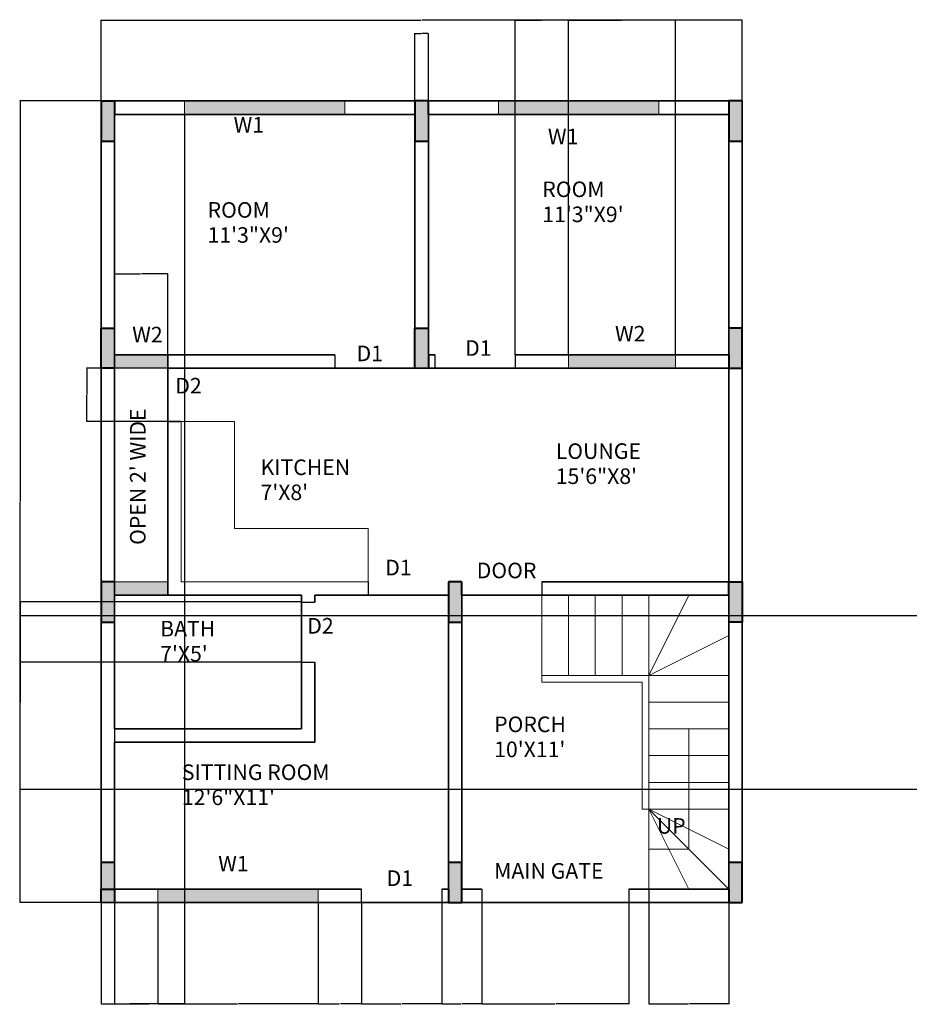
# Model space of a CAD drawing. Units: millimetres. Extents: x 1831 to 2754, y 1517 to 2450.
# Tile 1 of 4: x 1955 to 2355, y 1517 to 1959. Entities that reach past the tile are written whole.
import ezdxf

# ---------------------------------------------------------------- set-up
doc = ezdxf.new("R2010")
doc.units = ezdxf.units.MM
for name, color, linetype, lineweight in [('A-ANNO-DIMS', 2, 'Continuous', 18), ('A-ANNO-TEXT', 7, 'Continuous', 18), ('A-AREA-IDEN', 7, 'Continuous', 18), ('A-COLS', 7, 'Continuous', 40), ('A-DETL-REFP', 8, 'Continuous', 13), ('A-DOOR', 3, 'Continuous', 25), ('A-FLOR-CASE', 8, 'Continuous', 18), ('A-FLOR-STRS', 7, 'Continuous', 18), ('A-GLAZ', 4, 'Continuous', 18), ('A-WALL', 7, 'Continuous', 35)]:
    doc.layers.add(name, color=color, linetype=linetype, lineweight=lineweight)
doc.layers.add('A-COLS-PATT', color=18, linetype='Continuous', lineweight=13, true_color=0x000000)
doc.layers.add('A-GLAZ-PATT', color=252, linetype='Continuous', lineweight=13, true_color=0x939598)
doc.styles.get("Standard").update_dxf_attribs({"font": 'arial.ttf'})
doc.dimstyles.get("Standard").update_dxf_attribs({"dimtxt": 0.18, "dimasz": 0.18, "dimexe": 0.18, "dimexo": 0.0625, "dimgap": 0.09, "dimtad": 0, "dimtih": 1, "dimtoh": 1, "dimdec": 4, "dimzin": 0, "dimdsep": 46, "dimtxsty": 'Standard', "dimcen": 0.09, "dimadec": 0, "dimazin": 0, "dimtfac": 1, "dimtdec": 4, "dimtofl": 0, "dimtmove": 0, "dimatfit": 3, "dimfxl": 1, "dimtolj": 1, "dimtzin": 0, "dimarcsym": 0})

# ---------------------------------------------------------------- blocks, each defined once
blk = doc.blocks.new('*D22')
at = {"layer": 'A-ANNO-DIMS', "color": 0, "lineweight": -2, "transparency": 16777216}
for p, q in [((1991.57, 1922.44), (1991.57, 1958.89)), ((2279.57, 1922.44), (2279.57, 1958.89)), ((1991.75, 1958.71), (2135.28, 1958.71)), ((2279.39, 1958.71), (2135.86, 1958.71))]:
    blk.add_line(p, q, dxfattribs=at)
at = {"layer": 'A-ANNO-DIMS', "color": 0, "transparency": 16777216}
for points in [[(1991.75, 1958.74), (1991.75, 1958.68), (1991.57, 1958.71)], [(2279.39, 1958.74), (2279.39, 1958.68), (2279.57, 1958.71)]]:
    blk.add_solid(points, dxfattribs=at)
at = {"layer": 'Defpoints', "color": 0, "transparency": 16777216}
for p in [(2279.57, 1958.71), (1991.57, 1922.38), (2279.57, 1922.38)]:
    blk.add_point(p, dxfattribs=at)
at = {"layer": 'A-ANNO-DIMS', "color": 0, "transparency": 16777216, "insert": (2135.57, 1958.71), "char_height": 0.18, "attachment_point": 5}
blk.add_mtext('\\A1;288', dxfattribs=at)
blk = doc.blocks.new('*D23')
at = {"layer": 'A-ANNO-DIMS', "color": 0, "lineweight": -2, "transparency": 16777216}
for p, q in [((1991.51, 1922.38), (1955.06, 1922.38)), ((1955.24, 1922.2), (1955.24, 1742.56)), ((1955.24, 1562.56), (1955.24, 1742.2)), ((1991.51, 1562.38), (1955.06, 1562.38))]:
    blk.add_line(p, q, dxfattribs=at)
at = {"layer": 'A-ANNO-DIMS', "color": 0, "transparency": 16777216}
for points in [[(1955.21, 1922.2), (1955.27, 1922.2), (1955.24, 1922.38)], [(1955.21, 1562.56), (1955.27, 1562.56), (1955.24, 1562.38)]]:
    blk.add_solid(points, dxfattribs=at)
at = {"layer": 'Defpoints', "color": 0, "transparency": 16777216}
for p in [(1955.24, 1922.38), (1991.57, 1922.38), (1991.57, 1562.38)]:
    blk.add_point(p, dxfattribs=at)
at = {"layer": 'A-ANNO-DIMS', "color": 0, "transparency": 16777216, "insert": (1955.24, 1742.38), "char_height": 0.18, "attachment_point": 5}
blk.add_mtext('\\A1;360', dxfattribs=at)
blk = doc.blocks.new('*D24')
at = {"layer": 'A-ANNO-DIMS', "color": 0, "lineweight": -2, "transparency": 16777216}
for p, q in [((1991.57, 1562.32), (1991.57, 1516.71)), ((2017.07, 1562.32), (2017.07, 1516.71)), ((1991.75, 1516.89), (2003.99, 1516.89)), ((2016.89, 1516.89), (2004.64, 1516.89))]:
    blk.add_line(p, q, dxfattribs=at)
at = {"layer": 'A-ANNO-DIMS', "color": 0, "transparency": 16777216}
for points in [[(1991.75, 1516.92), (1991.75, 1516.86), (1991.57, 1516.89)], [(2016.89, 1516.92), (2016.89, 1516.86), (2017.07, 1516.89)]]:
    blk.add_solid(points, dxfattribs=at)
at = {"layer": 'Defpoints', "color": 0, "transparency": 16777216}
for p in [(1991.57, 1562.38), (2017.07, 1562.38), (2017.07, 1516.89)]:
    blk.add_point(p, dxfattribs=at)
at = {"layer": 'A-ANNO-DIMS', "color": 0, "transparency": 16777216, "insert": (2004.32, 1516.89), "char_height": 0.18, "attachment_point": 5}
blk.add_mtext('\\A1;25.5', dxfattribs=at)
blk = doc.blocks.new('*D25')
at = {"layer": 'A-ANNO-DIMS', "color": 0, "lineweight": -2, "transparency": 16777216}
for p, q in [((2017.07, 1562.32), (2017.07, 1516.71)), ((2089.07, 1562.32), (2089.07, 1516.71)), ((2017.25, 1516.89), (2052.85, 1516.89)), ((2088.89, 1516.89), (2053.29, 1516.89))]:
    blk.add_line(p, q, dxfattribs=at)
at = {"layer": 'A-ANNO-DIMS', "color": 0, "transparency": 16777216}
for points in [[(2017.25, 1516.92), (2017.25, 1516.86), (2017.07, 1516.89)], [(2088.89, 1516.92), (2088.89, 1516.86), (2089.07, 1516.89)]]:
    blk.add_solid(points, dxfattribs=at)
at = {"layer": 'Defpoints', "color": 0, "transparency": 16777216}
for p in [(2017.07, 1562.38), (2089.07, 1562.38), (2089.07, 1516.89)]:
    blk.add_point(p, dxfattribs=at)
at = {"layer": 'A-ANNO-DIMS', "color": 0, "transparency": 16777216, "insert": (2053.07, 1516.89), "char_height": 0.18, "attachment_point": 5}
blk.add_mtext('\\A1;72', dxfattribs=at)
blk = doc.blocks.new('*D26')
at = {"layer": 'A-ANNO-DIMS', "color": 0, "lineweight": -2, "transparency": 16777216}
for p, q in [((2089.07, 1562.32), (2089.07, 1516.71)), ((2108.57, 1562.32), (2108.57, 1516.71)), ((2089.25, 1516.89), (2098.5, 1516.89)), ((2108.39, 1516.89), (2099.13, 1516.89))]:
    blk.add_line(p, q, dxfattribs=at)
at = {"layer": 'A-ANNO-DIMS', "color": 0, "transparency": 16777216}
for points in [[(2089.25, 1516.92), (2089.25, 1516.86), (2089.07, 1516.89)], [(2108.39, 1516.92), (2108.39, 1516.86), (2108.57, 1516.89)]]:
    blk.add_solid(points, dxfattribs=at)
at = {"layer": 'Defpoints', "color": 0, "transparency": 16777216}
for p in [(2089.07, 1562.38), (2108.57, 1562.38), (2108.57, 1516.89)]:
    blk.add_point(p, dxfattribs=at)
at = {"layer": 'A-ANNO-DIMS', "color": 0, "transparency": 16777216, "insert": (2098.82, 1516.89), "char_height": 0.18, "attachment_point": 5}
blk.add_mtext('\\A1;19.5', dxfattribs=at)
blk = doc.blocks.new('*D27')
at = {"layer": 'A-ANNO-DIMS', "color": 0, "lineweight": -2, "transparency": 16777216}
for p, q in [((2108.57, 1562.32), (2108.57, 1516.71)), ((2144.57, 1562.32), (2144.57, 1516.71)), ((2108.75, 1516.89), (2126.35, 1516.89)), ((2144.39, 1516.89), (2126.79, 1516.89))]:
    blk.add_line(p, q, dxfattribs=at)
at = {"layer": 'A-ANNO-DIMS', "color": 0, "transparency": 16777216}
for points in [[(2108.75, 1516.92), (2108.75, 1516.86), (2108.57, 1516.89)], [(2144.39, 1516.92), (2144.39, 1516.86), (2144.57, 1516.89)]]:
    blk.add_solid(points, dxfattribs=at)
at = {"layer": 'Defpoints', "color": 0, "transparency": 16777216}
for p in [(2108.57, 1562.38), (2144.57, 1562.38), (2144.57, 1516.89)]:
    blk.add_point(p, dxfattribs=at)
at = {"layer": 'A-ANNO-DIMS', "color": 0, "transparency": 16777216, "insert": (2126.57, 1516.89), "char_height": 0.18, "attachment_point": 5}
blk.add_mtext('\\A1;36', dxfattribs=at)
blk = doc.blocks.new('*D28')
at = {"layer": 'A-ANNO-DIMS', "color": 0, "lineweight": -2, "transparency": 16777216}
for p, q in [((2144.57, 1562.32), (2144.57, 1516.71)), ((2162.57, 1562.32), (2162.57, 1516.71)), ((2144.75, 1516.89), (2153.36, 1516.89)), ((2162.39, 1516.89), (2153.78, 1516.89))]:
    blk.add_line(p, q, dxfattribs=at)
at = {"layer": 'A-ANNO-DIMS', "color": 0, "transparency": 16777216}
for points in [[(2144.75, 1516.92), (2144.75, 1516.86), (2144.57, 1516.89)], [(2162.39, 1516.92), (2162.39, 1516.86), (2162.57, 1516.89)]]:
    blk.add_solid(points, dxfattribs=at)
at = {"layer": 'Defpoints', "color": 0, "transparency": 16777216}
for p in [(2144.57, 1562.38), (2162.57, 1562.38), (2162.57, 1516.89)]:
    blk.add_point(p, dxfattribs=at)
at = {"layer": 'A-ANNO-DIMS', "color": 0, "transparency": 16777216, "insert": (2153.57, 1516.89), "char_height": 0.18, "attachment_point": 5}
blk.add_mtext('\\A1;18', dxfattribs=at)
blk = doc.blocks.new('*D29')
at = {"layer": 'A-ANNO-DIMS', "color": 0, "lineweight": -2, "transparency": 16777216}
for p, q in [((2162.57, 1562.32), (2162.57, 1516.71)), ((2228.57, 1562.32), (2228.57, 1516.71)), ((2162.75, 1516.89), (2195.35, 1516.89)), ((2228.39, 1516.89), (2195.79, 1516.89))]:
    blk.add_line(p, q, dxfattribs=at)
at = {"layer": 'A-ANNO-DIMS', "color": 0, "transparency": 16777216}
for points in [[(2162.75, 1516.92), (2162.75, 1516.86), (2162.57, 1516.89)], [(2228.39, 1516.92), (2228.39, 1516.86), (2228.57, 1516.89)]]:
    blk.add_solid(points, dxfattribs=at)
at = {"layer": 'Defpoints', "color": 0, "transparency": 16777216}
for p in [(2162.57, 1562.38), (2228.57, 1562.38), (2228.57, 1516.89)]:
    blk.add_point(p, dxfattribs=at)
at = {"layer": 'A-ANNO-DIMS', "color": 0, "transparency": 16777216, "insert": (2195.57, 1516.89), "char_height": 0.18, "attachment_point": 5}
blk.add_mtext('\\A1;66', dxfattribs=at)
blk = doc.blocks.new('*D30')
at = {"layer": 'A-ANNO-DIMS', "color": 0, "lineweight": -2, "transparency": 16777216}
for p, q in [((1997.57, 1916.32), (1997.57, 1516.71)), ((2029.07, 1916.32), (2029.07, 1516.71)), ((1997.75, 1516.89), (2012.99, 1516.89)), ((2028.89, 1516.89), (2013.64, 1516.89))]:
    blk.add_line(p, q, dxfattribs=at)
at = {"layer": 'A-ANNO-DIMS', "color": 0, "transparency": 16777216}
for points in [[(1997.75, 1516.92), (1997.75, 1516.86), (1997.57, 1516.89)], [(2028.89, 1516.92), (2028.89, 1516.86), (2029.07, 1516.89)]]:
    blk.add_solid(points, dxfattribs=at)
at = {"layer": 'Defpoints', "color": 0, "transparency": 16777216}
for p in [(1997.57, 1916.38), (2029.07, 1916.38), (2029.07, 1516.89)]:
    blk.add_point(p, dxfattribs=at)
at = {"layer": 'A-ANNO-DIMS', "color": 0, "transparency": 16777216, "insert": (2013.32, 1516.89), "char_height": 0.18, "attachment_point": 5}
blk.add_mtext('\\A1;31.5', dxfattribs=at)
blk = doc.blocks.new('*D31')
at = {"layer": 'A-ANNO-DIMS', "color": 0, "lineweight": -2, "transparency": 16777216}
for p, q in [((2177.57, 1808.44), (2177.57, 1958.89)), ((2201.57, 1808.44), (2201.57, 1958.89)), ((2177.75, 1958.71), (2189.35, 1958.71)), ((2201.39, 1958.71), (2189.79, 1958.71))]:
    blk.add_line(p, q, dxfattribs=at)
at = {"layer": 'A-ANNO-DIMS', "color": 0, "transparency": 16777216}
for points in [[(2177.75, 1958.74), (2177.75, 1958.68), (2177.57, 1958.71)], [(2201.39, 1958.74), (2201.39, 1958.68), (2201.57, 1958.71)]]:
    blk.add_solid(points, dxfattribs=at)
at = {"layer": 'Defpoints', "color": 0, "transparency": 16777216}
for p in [(2201.57, 1958.71), (2177.57, 1808.38), (2201.57, 1808.38)]:
    blk.add_point(p, dxfattribs=at)
at = {"layer": 'A-ANNO-DIMS', "color": 0, "transparency": 16777216, "insert": (2189.57, 1958.71), "char_height": 0.18, "attachment_point": 5}
blk.add_mtext('\\A1;24', dxfattribs=at)
blk = doc.blocks.new('*D32')
at = {"layer": 'A-ANNO-DIMS', "color": 0, "lineweight": -2, "transparency": 16777216}
for p, q in [((2201.57, 1808.44), (2201.57, 1958.89)), ((2249.57, 1808.44), (2249.57, 1958.89)), ((2201.75, 1958.71), (2225.35, 1958.71)), ((2249.39, 1958.71), (2225.79, 1958.71))]:
    blk.add_line(p, q, dxfattribs=at)
at = {"layer": 'A-ANNO-DIMS', "color": 0, "transparency": 16777216}
for points in [[(2201.75, 1958.74), (2201.75, 1958.68), (2201.57, 1958.71)], [(2249.39, 1958.74), (2249.39, 1958.68), (2249.57, 1958.71)]]:
    blk.add_solid(points, dxfattribs=at)
at = {"layer": 'Defpoints', "color": 0, "transparency": 16777216}
for p in [(2249.57, 1958.71), (2201.57, 1808.38), (2249.57, 1808.38)]:
    blk.add_point(p, dxfattribs=at)
at = {"layer": 'A-ANNO-DIMS', "color": 0, "transparency": 16777216, "insert": (2225.57, 1958.71), "char_height": 0.18, "attachment_point": 5}
blk.add_mtext('\\A1;48', dxfattribs=at)
blk = doc.blocks.new('*D33')
at = {"layer": 'A-ANNO-DIMS', "color": 0, "lineweight": -2, "transparency": 16777216}
for p, q in [((1997.57, 1808.44), (1997.57, 1844.89)), ((1997.75, 1844.71), (2009.35, 1844.71)), ((2021.39, 1844.71), (2009.79, 1844.71)), ((2021.57, 1808.44), (2021.57, 1844.89))]:
    blk.add_line(p, q, dxfattribs=at)
at = {"layer": 'A-ANNO-DIMS', "color": 0, "transparency": 16777216}
for points in [[(1997.75, 1844.74), (1997.75, 1844.68), (1997.57, 1844.71)], [(2021.39, 1844.74), (2021.39, 1844.68), (2021.57, 1844.71)]]:
    blk.add_solid(points, dxfattribs=at)
at = {"layer": 'Defpoints', "color": 0, "transparency": 16777216}
for p in [(2021.57, 1844.71), (1997.57, 1808.38), (2021.57, 1808.38)]:
    blk.add_point(p, dxfattribs=at)
at = {"layer": 'A-ANNO-DIMS', "color": 0, "transparency": 16777216, "insert": (2009.57, 1844.71), "char_height": 0.18, "attachment_point": 5}
blk.add_mtext('\\A1;24', dxfattribs=at)
blk = doc.blocks.new('*D34')
at = {"layer": 'A-ANNO-DIMS', "color": 0, "lineweight": -2, "transparency": 16777216}
for p, q in [((2021.51, 1802.38), (1985.06, 1802.38)), ((1985.24, 1802.2), (1985.24, 1790.56)), ((1985.24, 1778.56), (1985.24, 1790.2)), ((2021.51, 1778.38), (1985.06, 1778.38))]:
    blk.add_line(p, q, dxfattribs=at)
at = {"layer": 'A-ANNO-DIMS', "color": 0, "transparency": 16777216}
for points in [[(1985.21, 1802.2), (1985.27, 1802.2), (1985.24, 1802.38)], [(1985.21, 1778.56), (1985.27, 1778.56), (1985.24, 1778.38)]]:
    blk.add_solid(points, dxfattribs=at)
at = {"layer": 'Defpoints', "color": 0, "transparency": 16777216}
for p in [(1985.24, 1802.38), (2021.57, 1802.38), (2021.57, 1778.38)]:
    blk.add_point(p, dxfattribs=at)
at = {"layer": 'A-ANNO-DIMS', "color": 0, "transparency": 16777216, "insert": (1985.24, 1790.38), "char_height": 0.18, "attachment_point": 5}
blk.add_mtext('\\A1;24', dxfattribs=at)
blk = doc.blocks.new('*D35')
at = {"layer": 'A-ANNO-DIMS', "color": 0, "lineweight": -2, "transparency": 16777216}
for p, q in [((2081.51, 1697.38), (1955.06, 1697.38)), ((1955.24, 1697.2), (1955.24, 1684.06)), ((1955.24, 1670.56), (1955.24, 1683.7)), ((2081.51, 1670.38), (1955.06, 1670.38))]:
    blk.add_line(p, q, dxfattribs=at)
at = {"layer": 'A-ANNO-DIMS', "color": 0, "transparency": 16777216}
for points in [[(1955.21, 1697.2), (1955.27, 1697.2), (1955.24, 1697.38)], [(1955.21, 1670.56), (1955.27, 1670.56), (1955.24, 1670.38)]]:
    blk.add_solid(points, dxfattribs=at)
at = {"layer": 'Defpoints', "color": 0, "transparency": 16777216}
for p in [(1955.24, 1697.38), (2081.57, 1697.38), (2081.57, 1670.38)]:
    blk.add_point(p, dxfattribs=at)
at = {"layer": 'A-ANNO-DIMS', "color": 0, "transparency": 16777216, "insert": (1955.24, 1683.88), "char_height": 0.18, "attachment_point": 5}
blk.add_mtext('\\A1;27', dxfattribs=at)
blk = doc.blocks.new('*D36')
at = {"layer": 'A-ANNO-DIMS', "color": 0, "lineweight": -2, "transparency": 16777216}
for p, q in [((2237.57, 1568.32), (2237.57, 1516.71)), ((2273.57, 1568.32), (2273.57, 1516.71)), ((2237.75, 1516.89), (2255.35, 1516.89)), ((2273.39, 1516.89), (2255.79, 1516.89))]:
    blk.add_line(p, q, dxfattribs=at)
at = {"layer": 'A-ANNO-DIMS', "color": 0, "transparency": 16777216}
for points in [[(2237.75, 1516.92), (2237.75, 1516.86), (2237.57, 1516.89)], [(2273.39, 1516.92), (2273.39, 1516.86), (2273.57, 1516.89)]]:
    blk.add_solid(points, dxfattribs=at)
at = {"layer": 'Defpoints', "color": 0, "transparency": 16777216}
for p in [(2237.57, 1568.38), (2273.57, 1568.38), (2273.57, 1516.89)]:
    blk.add_point(p, dxfattribs=at)
at = {"layer": 'A-ANNO-DIMS', "color": 0, "transparency": 16777216, "insert": (2255.57, 1516.89), "char_height": 0.18, "attachment_point": 5}
blk.add_mtext('\\A1;36', dxfattribs=at)
blk = doc.blocks.new('*D37')
at = {"layer": 'A-ANNO-DIMS', "color": 0, "lineweight": -2, "transparency": 16777216}
for p, q in [((2132.57, 1916.44), (2132.57, 1952.89)), ((2132.75, 1952.71), (2135.42, 1952.71)), ((2138.39, 1952.71), (2135.72, 1952.71)), ((2138.57, 1916.44), (2138.57, 1952.89))]:
    blk.add_line(p, q, dxfattribs=at)
at = {"layer": 'A-ANNO-DIMS', "color": 0, "transparency": 16777216}
for points in [[(2132.75, 1952.74), (2132.75, 1952.68), (2132.57, 1952.71)], [(2138.39, 1952.74), (2138.39, 1952.68), (2138.57, 1952.71)]]:
    blk.add_solid(points, dxfattribs=at)
at = {"layer": 'Defpoints', "color": 0, "transparency": 16777216}
for p in [(2138.57, 1952.71), (2132.57, 1916.38), (2138.57, 1916.38)]:
    blk.add_point(p, dxfattribs=at)
at = {"layer": 'A-ANNO-DIMS', "color": 0, "transparency": 16777216, "insert": (2135.57, 1952.71), "char_height": 0.18, "attachment_point": 5}
blk.add_mtext('\\A1;6', dxfattribs=at)
blk = doc.blocks.new('*D44')
at = {"layer": 'A-ANNO-DIMS', "color": 0, "lineweight": -2, "transparency": 16777216}
for p, q in [((2627.54, 1691.22), (1955.06, 1691.22)), ((1955.24, 1691.04), (1955.24, 1652.4)), ((1955.24, 1613.4), (1955.24, 1652.03)), ((2627.54, 1613.22), (1955.06, 1613.22))]:
    blk.add_line(p, q, dxfattribs=at)
at = {"layer": 'A-ANNO-DIMS', "color": 0, "transparency": 16777216}
for points in [[(1955.21, 1691.04), (1955.27, 1691.04), (1955.24, 1691.22)], [(1955.21, 1613.4), (1955.27, 1613.4), (1955.24, 1613.22)]]:
    blk.add_solid(points, dxfattribs=at)
at = {"layer": 'Defpoints', "color": 0, "transparency": 16777216}
for p in [(1955.24, 1691.22), (2627.6, 1691.22), (2627.6, 1613.22)]:
    blk.add_point(p, dxfattribs=at)
at = {"layer": 'A-ANNO-DIMS', "color": 0, "transparency": 16777216, "insert": (1955.24, 1652.22), "char_height": 0.18, "attachment_point": 5}
blk.add_mtext('\\A1;78', dxfattribs=at)

msp = doc.modelspace()

# ---------------------------------------------------------------- hatches: boundary and pattern name
at = {"layer": 'A-COLS-PATT'}
h = msp.add_hatch(color=256, dxfattribs=at)
h.dxf.hatch_style = 1
h.paths.add_polyline_path([(1997.569, 1916.378), (1997.569, 1922.378), (1991.569, 1922.378), (1991.569, 1904.378), (1997.569, 1904.378)])
h.paths.add_polyline_path([(1997.569, 1820.378), (1991.569, 1820.378), (1991.569, 1802.378), (1997.569, 1802.378), (1997.569, 1808.378)])
h.paths.add_polyline_path([(2138.569, 1820.378), (2132.569, 1820.378), (2132.569, 1802.378), (2138.569, 1802.378), (2138.569, 1808.378)])
h.paths.add_polyline_path([(2138.569, 1916.378), (2138.569, 1922.378), (2132.569, 1922.378), (2132.569, 1904.378), (2138.569, 1904.378)])
h.paths.add_polyline_path([(2279.569, 1922.378), (2273.569, 1922.378), (2273.569, 1904.378), (2279.569, 1904.378)])
h.paths.add_polyline_path([(2279.569, 1820.378), (2273.569, 1820.378), (2273.569, 1808.378), (2273.569, 1802.378), (2279.569, 1802.378)])
h.paths.add_polyline_path([(1997.569, 1706.378), (1991.569, 1706.378), (1991.569, 1688.378), (1997.569, 1688.378), (1997.569, 1700.378)])
h.paths.add_polyline_path([(2153.569, 1700.378), (2153.569, 1706.378), (2147.569, 1706.378), (2147.569, 1688.378), (2153.569, 1688.378)])
h.paths.add_polyline_path([(2279.569, 1706.378), (2273.569, 1706.378), (2273.569, 1700.378), (2273.569, 1688.378), (2279.569, 1688.378)])
h.paths.add_polyline_path([(2435.602, 1907.216), (2435.602, 1913.216), (2429.602, 1913.216), (2429.602, 1895.216), (2435.602, 1895.216)])
h.paths.add_polyline_path([(2435.602, 1811.216), (2429.602, 1811.216), (2429.602, 1793.216), (2435.602, 1793.216), (2435.602, 1799.216)])
h.paths.add_polyline_path([(2576.602, 1811.216), (2570.602, 1811.216), (2570.602, 1799.216), (2570.602, 1793.216), (2576.602, 1793.216)])
h.paths.add_polyline_path([(2576.602, 1907.216), (2570.602, 1907.216), (2570.602, 1895.216), (2576.602, 1895.216)])
h.paths.add_polyline_path([(2576.602, 1913.216), (2570.602, 1913.216), (2570.602, 1907.216), (2576.602, 1907.216)])
h.paths.add_polyline_path([(2717.602, 1811.216), (2711.602, 1811.216), (2711.602, 1799.216), (2711.602, 1793.216), (2717.602, 1793.216)])
h.paths.add_polyline_path([(2435.602, 1691.216), (2435.602, 1697.216), (2429.602, 1697.216), (2429.602, 1679.216), (2435.602, 1679.216)])
h.paths.add_polyline_path([(2591.602, 1691.216), (2591.602, 1697.216), (2585.602, 1697.216), (2585.602, 1691.216), (2585.602, 1679.216), (2591.602, 1679.216)])
h.paths.add_polyline_path([(2717.602, 1697.216), (2711.602, 1697.216), (2711.602, 1691.216), (2711.602, 1679.216), (2717.602, 1679.216)])
h.paths.add_polyline_path([(2717.602, 1913.216), (2711.602, 1913.216), (2711.602, 1907.216), (2711.602, 1895.216), (2717.602, 1895.216)])
h.paths.add_polyline_path([(1997.569, 1580.378), (1991.569, 1580.378), (1991.569, 1568.378), (1997.569, 1568.378)])
h.paths.add_polyline_path([(1997.569, 1568.378), (1991.569, 1568.378), (1991.569, 1562.378), (1997.569, 1562.378)])
h.paths.add_polyline_path([(2153.569, 1580.378), (2147.569, 1580.378), (2147.569, 1568.378), (2147.569, 1562.378), (2153.569, 1562.378)])
h.paths.add_polyline_path([(2279.569, 1580.378), (2273.569, 1580.378), (2273.569, 1568.378), (2273.569, 1562.378), (2279.569, 1562.378)])
h.paths.add_polyline_path([(2435.602, 1571.216), (2429.602, 1571.216), (2429.602, 1553.216), (2435.602, 1553.216)])
h.paths.add_polyline_path([(2717.602, 1571.216), (2711.602, 1571.216), (2711.602, 1559.216), (2711.602, 1553.216), (2717.602, 1553.216)])
h.paths.add_polyline_path([(2591.602, 1571.216), (2585.602, 1571.216), (2585.602, 1559.216), (2585.602, 1553.216), (2591.602, 1553.216)])
at = {"layer": 'A-GLAZ-PATT'}
h = msp.add_hatch(color=256, dxfattribs=at)
h.dxf.hatch_style = 1
h.paths.add_polyline_path([(2021.569, 1808.378), (1997.569, 1808.378), (1997.569, 1802.378), (2021.569, 1802.378)])
h.paths.add_polyline_path([(2101.069, 1922.378), (2029.069, 1922.378), (2029.069, 1916.378), (2065.069, 1916.378), (2101.069, 1916.378)])
h.paths.add_polyline_path([(2242.069, 1922.378), (2170.069, 1922.378), (2170.069, 1916.378), (2206.069, 1916.378), (2242.069, 1916.378)])
h.paths.add_polyline_path([(2249.569, 1808.378), (2225.569, 1808.378), (2201.569, 1808.378), (2201.569, 1802.378), (2249.569, 1802.378)])
h.paths.add_polyline_path([(2089.069, 1568.378), (2017.069, 1568.378), (2017.069, 1562.378), (2089.069, 1562.378)])
h.paths.add_polyline_path([(2021.569, 1706.378), (1997.569, 1706.378), (1997.569, 1700.378), (2021.569, 1700.378)])

# ---------------------------------------------------------------- linework, layer by layer
at = {"layer": 'A-COLS'}
for p, q in [((1991.569, 1922.378), (1997.569, 1922.378)), ((1991.569, 1922.378), (1991.569, 1904.378)), ((1997.569, 1922.378), (1997.569, 1916.378)), ((2138.569, 1922.378), (2132.569, 1922.378)), ((2132.569, 1922.378), (2132.569, 1904.378)), ((2138.569, 1916.378), (2138.569, 1922.378)), ((2279.569, 1922.378), (2273.569, 1922.378)), ((2273.569, 1922.378), (2273.569, 1904.378)), ((1991.569, 1904.378), (1997.569, 1904.378)), ((2132.569, 1904.378), (2138.569, 1904.378)), ((2273.569, 1904.378), (2279.569, 1904.378)), ((1991.569, 1802.378), (1991.569, 1820.378)), ((1991.569, 1820.378), (1997.569, 1820.378)), ((2132.569, 1802.378), (2132.569, 1820.378)), ((2132.569, 1820.378), (2138.569, 1820.378)), ((2279.569, 1820.378), (2273.569, 1820.378)), ((2279.569, 1802.378), (2279.569, 1820.378)), ((2132.569, 1802.378), (2132.569, 1808.378)), ((2138.569, 1808.378), (2138.569, 1802.378)), ((2273.569, 1808.378), (2273.569, 1802.378)), ((1997.569, 1802.378), (1991.569, 1802.378)), ((2273.569, 1802.378), (2279.569, 1802.378)), ((1997.569, 1706.378), (1991.569, 1706.378)), ((1991.569, 1706.378), (1991.569, 1688.378)), ((2153.569, 1706.378), (2147.569, 1706.378)), ((2147.569, 1706.378), (2147.569, 1688.378)), ((2153.569, 1706.378), (2147.569, 1706.378)), ((2153.569, 1700.378), (2153.569, 1706.378)), ((2273.569, 1700.378), (2273.569, 1706.378)), ((2273.569, 1706.378), (2279.569, 1706.378)), ((2279.569, 1706.378), (2279.569, 1688.378)), ((1991.569, 1688.378), (1997.569, 1688.378)), ((2147.569, 1688.378), (2153.569, 1688.378)), ((2279.569, 1688.378), (2273.569, 1688.378)), ((1997.569, 1580.378), (1991.569, 1580.378)), ((2153.569, 1580.378), (2147.569, 1580.378)), ((2153.569, 1562.378), (2153.569, 1580.378)), ((2279.569, 1580.378), (2273.569, 1580.378)), ((2279.569, 1562.378), (2279.569, 1580.378)), ((1991.569, 1562.378), (1991.569, 1568.378)), ((1991.569, 1568.378), (1997.569, 1568.378)), ((1997.569, 1568.378), (1997.569, 1562.378)), ((2147.569, 1568.378), (2147.569, 1562.378)), ((2273.569, 1568.378), (2273.569, 1562.378)), ((2147.569, 1562.378), (2153.569, 1562.378)), ((2273.569, 1562.378), (2279.569, 1562.378))]:
    msp.add_line(p, q, dxfattribs=at)
at = {"layer": 'A-DETL-REFP'}
for p in [(2201.569, 1664.378), (2213.569, 1664.378), (2225.569, 1664.378)]:
    msp.add_point(p, dxfattribs=at)
at = {"layer": 'A-DOOR'}
for p, q in [((2096.569, 1808.378), (2096.569, 1802.378)), ((2141.569, 1802.378), (2141.569, 1808.378)), ((2177.569, 1808.378), (2177.569, 1802.378)), ((2096.569, 1802.378), (2132.569, 1802.378)), ((2111.569, 1706.378), (2111.569, 1700.378)), ((2189.569, 1706.378), (2189.569, 1700.378)), ((2081.569, 1697.378), (2087.569, 1697.378)), ((2081.569, 1697.378), (2081.569, 1673.378)), ((2081.569, 1670.378), (2087.569, 1670.378)), ((2108.569, 1562.378), (2108.569, 1568.378)), ((2144.569, 1568.378), (2144.569, 1562.378)), ((2162.569, 1568.378), (2162.569, 1562.378)), ((2228.569, 1568.378), (2228.569, 1562.378)), ((2144.569, 1562.378), (2108.569, 1562.378))]:
    msp.add_line(p, q, dxfattribs=at)
at = {"layer": 'A-FLOR-CASE'}
for p, q in [((2027.569, 1778.378), (2027.569, 1706.378)), ((2051.569, 1778.378), (2027.569, 1778.378)), ((2051.569, 1730.378), (2051.569, 1778.378)), ((2111.569, 1730.378), (2051.569, 1730.378)), ((2111.569, 1730.378), (2111.569, 1706.378)), ((2111.569, 1706.378), (2111.569, 1730.378)), ((2027.569, 1706.378), (2111.569, 1706.378)), ((2027.569, 1706.378), (2111.569, 1706.378))]:
    msp.add_line(p, q, dxfattribs=at)
at = {"layer": 'A-FLOR-STRS'}
for p, q in [((2189.569, 1700.378), (2189.569, 1664.378)), ((2201.569, 1664.378), (2201.569, 1700.378)), ((2201.569, 1700.378), (2201.569, 1664.378)), ((2213.569, 1664.378), (2213.569, 1700.378)), ((2213.569, 1700.378), (2213.569, 1664.378)), ((2225.569, 1664.378), (2225.569, 1700.378)), ((2237.569, 1568.378), (2237.569, 1700.378)), ((2237.569, 1700.378), (2237.569, 1664.378)), ((2237.569, 1700.378), (2273.569, 1700.378)), ((2237.569, 1664.378), (2255.569, 1700.378)), ((2255.569, 1700.378), (2237.569, 1664.378)), ((2273.569, 1700.378), (2273.569, 1664.378)), ((2237.569, 1664.378), (2273.569, 1682.378)), ((2237.569, 1664.378), (2189.569, 1664.378)), ((2189.569, 1664.378), (2189.569, 1661.378)), ((2201.569, 1664.378), (2213.569, 1664.378)), ((2213.569, 1664.378), (2225.569, 1664.378)), ((2237.569, 1664.378), (2273.569, 1664.378)), ((2273.569, 1664.378), (2237.569, 1664.378)), ((2189.569, 1661.378), (2234.569, 1661.378)), ((2234.569, 1661.378), (2234.569, 1604.378)), ((2273.569, 1652.378), (2237.569, 1652.378)), ((2273.569, 1640.378), (2237.569, 1640.378)), ((2255.569, 1604.378), (2255.569, 1640.378)), ((2273.569, 1628.378), (2237.569, 1628.378)), ((2273.569, 1616.378), (2237.569, 1616.378)), ((2234.569, 1604.378), (2237.569, 1604.378)), ((2273.569, 1604.378), (2237.569, 1604.378)), ((2237.569, 1568.378), (2237.569, 1604.378)), ((2237.569, 1604.378), (2273.569, 1604.378)), ((2237.569, 1604.378), (2273.569, 1586.378)), ((2273.569, 1586.378), (2237.569, 1604.378)), ((2237.569, 1604.378), (2255.569, 1568.378)), ((2237.569, 1604.378), (2273.569, 1568.378)), ((2255.569, 1586.378), (2255.569, 1604.378)), ((2273.569, 1604.378), (2273.569, 1568.378)), ((2237.569, 1586.378), (2255.569, 1586.378)), ((2273.569, 1568.378), (2237.569, 1568.378))]:
    msp.add_line(p, q, dxfattribs=at)
at = {"layer": 'A-GLAZ'}
for p, q in [((2029.069, 1916.378), (2029.069, 1922.378)), ((2029.069, 1922.378), (2101.069, 1922.378)), ((2101.069, 1922.378), (2101.069, 1916.378)), ((2170.069, 1916.378), (2170.069, 1922.378)), ((2170.069, 1922.378), (2242.069, 1922.378)), ((2242.069, 1922.378), (2242.069, 1916.378)), ((2065.069, 1916.378), (2029.069, 1916.378)), ((2206.069, 1916.378), (2170.069, 1916.378)), ((1997.569, 1808.378), (1997.569, 1802.378)), ((2021.569, 1808.378), (1997.569, 1808.378)), ((2225.569, 1808.378), (2201.569, 1808.378)), ((2201.569, 1808.378), (2201.569, 1802.378)), ((2249.569, 1802.378), (2249.569, 1808.378)), ((1997.569, 1802.378), (2021.569, 1802.378)), ((2201.569, 1802.378), (2249.569, 1802.378)), ((2021.569, 1706.378), (1997.569, 1706.378)), ((2021.569, 1706.378), (2021.569, 1700.378)), ((2053.069, 1568.378), (2017.069, 1568.378)), ((2017.069, 1568.378), (2017.069, 1562.378)), ((2089.069, 1562.378), (2089.069, 1568.378)), ((2017.069, 1562.378), (2089.069, 1562.378))]:
    msp.add_line(p, q, dxfattribs=at)
at = {"layer": 'A-WALL'}
for p, q in [((1991.569, 1922.378), (2279.569, 1922.378)), ((1991.569, 1562.378), (1991.569, 1922.378)), ((2279.569, 1922.378), (2279.569, 1562.378)), ((1997.569, 1916.378), (2132.569, 1916.378)), ((1997.569, 1808.378), (1997.569, 1916.378)), ((1997.569, 1916.378), (2132.569, 1916.378)), ((1997.569, 1916.378), (2132.569, 1916.378)), ((2132.569, 1916.378), (2065.069, 1916.378)), ((2132.569, 1916.378), (2132.569, 1808.378)), ((2138.569, 1916.378), (2273.569, 1916.378)), ((2138.569, 1808.378), (2138.569, 1916.378)), ((2138.569, 1916.378), (2138.569, 1808.378)), ((2138.569, 1916.378), (2273.569, 1916.378)), ((2273.569, 1916.378), (2206.069, 1916.378)), ((2273.569, 1916.378), (2273.569, 1808.378)), ((2096.569, 1808.378), (1997.569, 1808.378)), ((1997.569, 1808.378), (1997.569, 1700.378)), ((2021.569, 1700.378), (2021.569, 1808.378)), ((2138.569, 1808.378), (2141.569, 1808.378)), ((2141.569, 1808.378), (2138.569, 1808.378)), ((2273.569, 1808.378), (2177.569, 1808.378)), ((2177.569, 1808.378), (2273.569, 1808.378)), ((2177.569, 1808.378), (2273.569, 1808.378)), ((2273.569, 1808.378), (2225.569, 1808.378)), ((1997.569, 1706.378), (1997.569, 1802.378)), ((2021.569, 1802.378), (2021.569, 1706.378)), ((2021.569, 1802.378), (2021.569, 1778.378)), ((2111.569, 1802.378), (2021.569, 1802.378)), ((2273.569, 1802.378), (2111.569, 1802.378)), ((2273.569, 1802.378), (2111.569, 1802.378)), ((2138.569, 1802.378), (2141.569, 1802.378)), ((2273.569, 1802.378), (2273.569, 1706.378)), ((2021.569, 1778.378), (2027.569, 1778.378)), ((2273.569, 1706.378), (2189.569, 1706.378)), ((1997.569, 1700.378), (1997.569, 1640.378)), ((2081.569, 1700.378), (1997.569, 1700.378)), ((2081.569, 1640.378), (2081.569, 1700.378)), ((2081.569, 1700.378), (2081.569, 1697.378)), ((2147.569, 1700.378), (2087.569, 1700.378)), ((2087.569, 1700.378), (2087.569, 1697.378)), ((2147.569, 1568.378), (2147.569, 1700.378)), ((2153.569, 1700.378), (2273.569, 1700.378)), ((2153.569, 1568.378), (2153.569, 1700.378)), ((2153.569, 1700.378), (2273.569, 1700.378)), ((2273.569, 1700.378), (2273.569, 1568.378)), ((2087.569, 1670.378), (2087.569, 1640.378)), ((1997.569, 1640.378), (2081.569, 1640.378)), ((2087.569, 1640.378), (2087.569, 1634.378)), ((2003.569, 1634.378), (1997.569, 1634.378)), ((1997.569, 1634.378), (1997.569, 1568.378)), ((2087.569, 1634.378), (2003.569, 1634.378)), ((1997.569, 1562.378), (1997.569, 1580.378)), ((1997.569, 1568.378), (2108.569, 1568.378)), ((1997.569, 1568.378), (2108.569, 1568.378)), ((2108.569, 1568.378), (2053.069, 1568.378)), ((2147.569, 1568.378), (2144.569, 1568.378)), ((2144.569, 1568.378), (2147.569, 1568.378)), ((2153.569, 1568.378), (2162.569, 1568.378)), ((2162.569, 1568.378), (2153.569, 1568.378)), ((2273.569, 1568.378), (2228.569, 1568.378)), ((2231.569, 1568.378), (2228.569, 1568.378)), ((2237.569, 1568.378), (2231.569, 1568.378)), ((2273.569, 1568.378), (2237.569, 1568.378)), ((2279.569, 1562.378), (1991.569, 1562.378))]:
    msp.add_line(p, q, dxfattribs=at)

# ---------------------------------------------------------------- texts
at = {"layer": 'A-ANNO-TEXT'}
for s, p in [('W1', (2051.109, 1908.207)), ('W1', (2192.264, 1902.92)), ('W2', (2005.567, 1813.976)), ('W2', (2222.393, 1814.379)), ('D1', (2155.088, 1807.936)), ('D1', (2106.322, 1805.52)), ('D2', (2024.912, 1791.023)), ('D1', (2119.204, 1709.337)), ('DOOR', (2160.3, 1708.034)), ('D2', (2084.174, 1683.19)), ('UP', (2241.188, 1593.318)), ('W1', (2044.187, 1576.372)), ('MAIN GATE', (2168.128, 1573.113)), ('D1', (2119.856, 1569.854))]:
    msp.add_text(s, height=7, dxfattribs=at).set_placement(p)
msp.add_text("OPEN 2' WIDE", height=7, rotation=90, dxfattribs=at).set_placement((2011.571, 1723.025))
at = {"layer": 'A-AREA-IDEN'}
for s, p in [('ROOM', (2189.748, 1879.213)), ('ROOM', (2039.421, 1869.951)), ('11\'3"X9\'', (2189.748, 1867.968)), ('11\'3"X9\'', (2039.421, 1858.706)), ('LOUNGE', (2195.793, 1761.626)), ('KITCHEN', (2063.199, 1754.377)), ('15\'6"X8\'', (2195.793, 1750.381)), ("7'X8'", (2063.199, 1743.133)), ('BATH', (2018.118, 1681.916)), ("7'X5'", (2018.118, 1670.671)), ('PORCH', (2168.128, 1638.944)), ("10'X11'", (2168.128, 1627.699)), ('SITTING ROOM', (2027.879, 1617.434)), ('12\'6"X11\'', (2027.879, 1606.19))]:
    msp.add_text(s, height=7, dxfattribs=at).set_placement(p)

# ---------------------------------------------------------------- dimensions: what is measured, and where the dimension line sits
at = {"layer": 'A-ANNO-DIMS'}
for base, p1, p2, override, picture, middle in [((2279.569, 1958.708), (1991.569, 1922.378), (2279.569, 1922.378), {"dimdec": 0, "dimlfac": 1, "dimrnd": 0, "dimzin": 0, "dimdsep": 46, "dimlunit": 2}, '*D22', (2135.569, 1958.708)), ((2201.569, 1958.708), (2177.569, 1808.378), (2201.569, 1808.378), {"dimdec": 0, "dimlfac": 1, "dimrnd": 0, "dimzin": 0, "dimdsep": 46, "dimlunit": 2}, '*D31', (2189.569, 1958.708)), ((2249.569, 1958.708), (2201.569, 1808.378), (2249.569, 1808.378), {"dimdec": 0, "dimlfac": 1, "dimrnd": 0, "dimzin": 0, "dimdsep": 46, "dimlunit": 2}, '*D32', (2225.569, 1958.708)), ((2138.569, 1952.708), (2132.569, 1916.378), (2138.569, 1916.378), {"dimdec": 0, "dimlfac": 1, "dimrnd": 0, "dimzin": 0, "dimdsep": 46, "dimlunit": 2}, '*D37', (2135.569, 1952.708)), ((2029.069, 1516.886), (1997.569, 1916.378), (2029.069, 1916.378), {"dimdec": 1, "dimlfac": 1, "dimrnd": 0, "dimzin": 0, "dimdsep": 46, "dimlunit": 2}, '*D30', (2013.319, 1516.886)), ((2021.569, 1844.708), (1997.569, 1808.378), (2021.569, 1808.378), {"dimdec": 0, "dimlfac": 1, "dimrnd": 0, "dimzin": 0, "dimdsep": 46, "dimlunit": 2}, '*D33', (2009.569, 1844.708)), ((2273.569, 1516.886), (2237.569, 1568.378), (2273.569, 1568.378), {"dimdec": 0, "dimlfac": 1, "dimrnd": 0, "dimzin": 0, "dimdsep": 46, "dimlunit": 2}, '*D36', (2255.569, 1516.886)), ((2017.069, 1516.886), (1991.569, 1562.378), (2017.069, 1562.378), {"dimdec": 1, "dimlfac": 1, "dimrnd": 0, "dimzin": 0, "dimdsep": 46, "dimlunit": 2}, '*D24', (2004.319, 1516.886)), ((2089.069, 1516.886), (2017.069, 1562.378), (2089.069, 1562.378), {"dimdec": 0, "dimlfac": 1, "dimrnd": 0, "dimzin": 0, "dimdsep": 46, "dimlunit": 2}, '*D25', (2053.069, 1516.886)), ((2108.569, 1516.886), (2089.069, 1562.378), (2108.569, 1562.378), {"dimdec": 1, "dimlfac": 1, "dimrnd": 0, "dimzin": 0, "dimdsep": 46, "dimlunit": 2}, '*D26', (2098.819, 1516.886)), ((2144.569, 1516.886), (2108.569, 1562.378), (2144.569, 1562.378), {"dimdec": 0, "dimlfac": 1, "dimrnd": 0, "dimzin": 0, "dimdsep": 46, "dimlunit": 2}, '*D27', (2126.569, 1516.886)), ((2162.569, 1516.886), (2144.569, 1562.378), (2162.569, 1562.378), {"dimdec": 0, "dimlfac": 1, "dimrnd": 0, "dimzin": 0, "dimdsep": 46, "dimlunit": 2}, '*D28', (2153.569, 1516.886)), ((2228.569, 1516.886), (2162.569, 1562.378), (2228.569, 1562.378), {"dimdec": 0, "dimlfac": 1, "dimrnd": 0, "dimzin": 0, "dimdsep": 46, "dimlunit": 2}, '*D29', (2195.569, 1516.886))]:
    dim = msp.add_linear_dim(base=base, p1=p1, p2=p2, dimstyle='Standard', override=override, dxfattribs=at)
    dim.commit()
    dim.dimension.update_dxf_attribs({"geometry": picture, "text_midpoint": middle})
for base, p1, p2, picture, middle in [((1955.239, 1922.378), (1991.569, 1562.378), (1991.569, 1922.378), '*D23', (1955.239, 1742.378)), ((1985.239, 1802.378), (2021.569, 1778.378), (2021.569, 1802.378), '*D34', (1985.239, 1790.378)), ((1955.239, 1697.378), (2081.569, 1670.378), (2081.569, 1697.378), '*D35', (1955.239, 1683.878)), ((1955.239, 1691.216), (2627.602, 1613.216), (2627.602, 1691.216), '*D44', (1955.239, 1652.216))]:
    dim = msp.add_linear_dim(base=base, p1=p1, p2=p2, angle=90, dimstyle='Standard', override={"dimdec": 0, "dimlfac": 1, "dimrnd": 0, "dimzin": 0, "dimdsep": 46, "dimlunit": 2}, dxfattribs=at)
    dim.commit()
    dim.dimension.update_dxf_attribs({"geometry": picture, "text_midpoint": middle})

doc.saveas('drawing.dxf')
